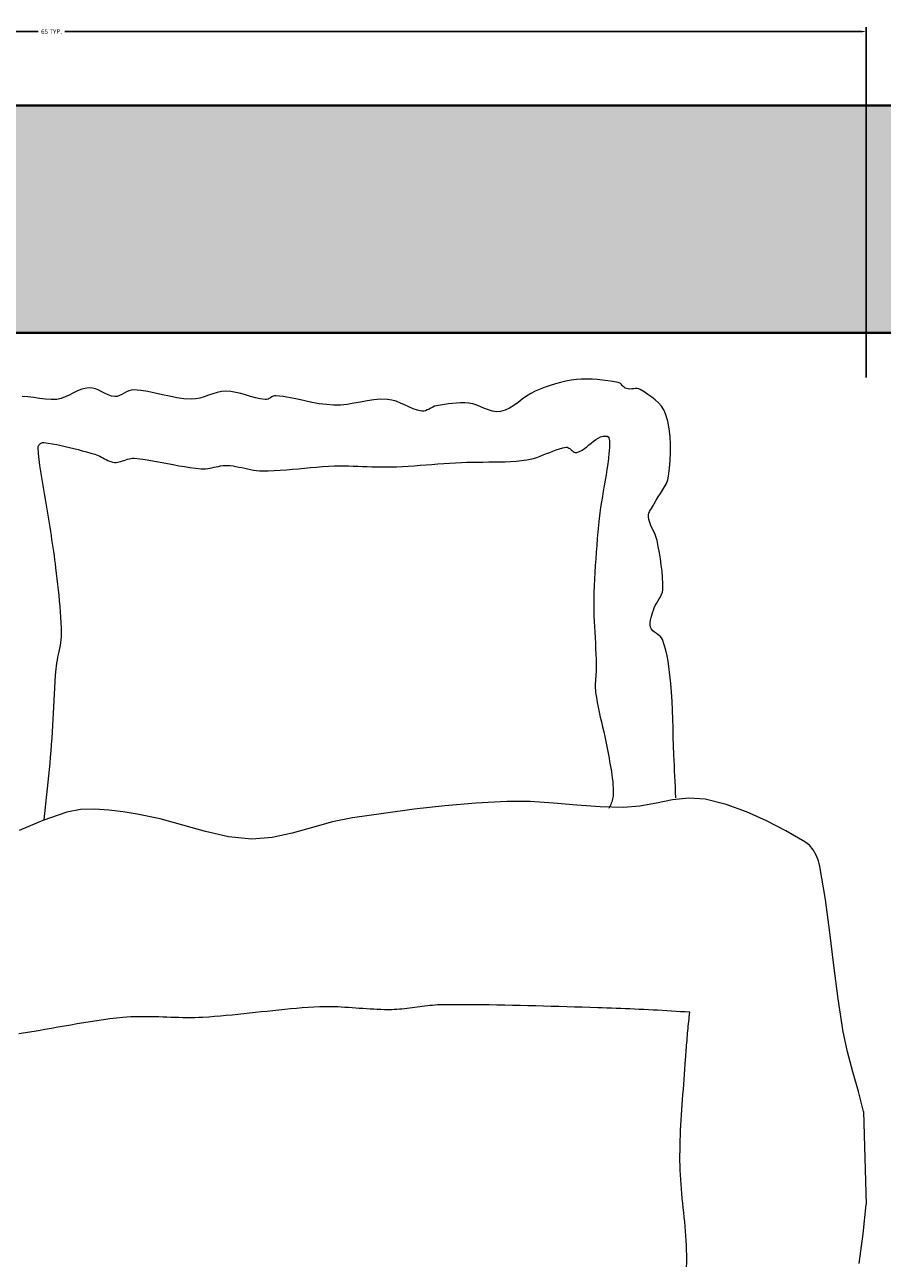
# Model space of a CAD drawing. Units: inches. Extents: x 1441 to 2460, y 1648 to 2683.
# Tile 28 of 35: x 1840 to 1874, y 2253 to 2302. Entities that reach past the tile are written whole.
import ezdxf

# ---------------------------------------------------------------- set-up
doc = ezdxf.new("R2010")
doc.units = ezdxf.units.IN
for name, color, linetype, lineweight in [('A-ANNO-DIMS', 2, 'Continuous', 18), ('A-FURN', 8, 'Continuous', 15), ('A-WALL', 7, 'Continuous', 40)]:
    doc.layers.add(name, color=color, linetype=linetype, lineweight=lineweight)
doc.layers.add('A-WALL-PATT', color=251, linetype='Continuous', lineweight=13, true_color=0x636466)
doc.styles.get("Standard").update_dxf_attribs({"font": 'arial.ttf'})
doc.dimstyles.get("Standard").update_dxf_attribs({"dimtxt": 0.18, "dimasz": 0.18, "dimexe": 0.18, "dimexo": 0.0625, "dimgap": 0.09, "dimtad": 0, "dimtih": 1, "dimtoh": 1, "dimdec": 4, "dimzin": 0, "dimdsep": 46, "dimtxsty": 'Standard', "dimcen": 0.09, "dimadec": 0, "dimazin": 0, "dimtfac": 1, "dimtdec": 4, "dimtofl": 0, "dimtmove": 0, "dimatfit": 3, "dimfxl": 1, "dimtolj": 1, "dimtzin": 0, "dimarcsym": 0})

# ---------------------------------------------------------------- blocks, each defined once
blk = doc.blocks.new('BED-DOUBLE-PLAN')
for p, q in [((53.027, 91.67), (52.818, 91.642)), ((53.234, 91.686), (53.027, 91.67)), ((53.441, 91.69), (53.234, 91.686)), ((53.649, 91.684), (53.441, 91.69)), ((53.857, 91.67), (53.649, 91.684)), ((33.253, 91.205), (33.099, 91.129)), ((33.41, 91.271), (33.253, 91.205)), ((33.569, 91.32), (33.41, 91.271)), ((33.735, 91.343), (33.569, 91.32)), ((33.867, 91.333), (33.735, 91.343)), ((33.995, 91.298), (33.867, 91.333)), ((34.121, 91.245), (33.995, 91.298)), ((34.245, 91.181), (34.121, 91.245)), ((34.37, 91.117), (34.245, 91.181)), ((35.307, 91.222), (35.216, 91.178)), ((35.4, 91.252), (35.307, 91.222)), ((35.496, 91.261), (35.4, 91.252)), ((35.784, 91.238), (35.496, 91.261)), ((36.07, 91.194), (35.784, 91.238)), ((36.354, 91.135), (36.07, 91.194)), ((38.983, 91.195), (38.81, 91.159)), ((39.158, 91.208), (38.983, 91.195)), ((39.356, 91.195), (39.158, 91.208)), ((39.551, 91.161), (39.356, 91.195)), ((51.403, 91.204), (51.224, 91.115)), ((51.599, 91.285), (51.403, 91.204)), ((51.797, 91.361), (51.599, 91.285)), ((51.997, 91.432), (51.797, 91.361)), ((52.2, 91.497), (51.997, 91.432)), ((52.404, 91.554), (52.2, 91.497)), ((52.61, 91.603), (52.404, 91.554)), ((52.818, 91.642), (52.61, 91.603)), ((54.065, 91.648), (53.857, 91.67)), ((54.272, 91.619), (54.065, 91.648)), ((54.478, 91.587), (54.272, 91.619)), ((54.683, 91.551), (54.478, 91.587)), ((54.729, 91.535), (54.683, 91.551)), ((54.771, 91.509), (54.729, 91.535)), ((54.81, 91.475), (54.771, 91.509)), ((54.847, 91.437), (54.81, 91.475)), ((54.884, 91.398), (54.847, 91.437)), ((54.922, 91.361), (54.884, 91.398)), ((54.963, 91.331), (54.922, 91.361)), ((55.008, 91.31), (54.963, 91.331)), ((55.076, 91.296), (55.008, 91.31)), ((55.147, 91.294), (55.076, 91.296)), ((55.219, 91.299), (55.147, 91.294)), ((55.292, 91.306), (55.219, 91.299)), ((55.364, 91.311), (55.292, 91.306)), ((55.433, 91.31), (55.364, 91.311)), ((55.499, 91.298), (55.433, 91.31)), ((55.56, 91.27), (55.499, 91.298)), ((55.709, 91.176), (55.56, 91.27)), ((31.32, 90.99), (31.094, 91.001)), ((31.549, 90.959), (31.32, 90.99)), ((31.78, 90.922), (31.549, 90.959)), ((32.011, 90.889), (31.78, 90.922)), ((32.24, 90.873), (32.011, 90.889)), ((32.466, 90.885), (32.24, 90.873)), ((32.63, 90.922), (32.466, 90.885)), ((32.789, 90.98), (32.63, 90.922)), ((32.945, 91.051), (32.789, 90.98)), ((33.099, 91.129), (32.945, 91.051)), ((34.495, 91.058), (34.37, 91.117)), ((34.624, 91.015), (34.495, 91.058)), ((34.756, 90.994), (34.624, 91.015)), ((34.852, 91.003), (34.756, 90.994)), ((34.945, 91.032), (34.852, 91.003)), ((35.036, 91.076), (34.945, 91.032)), ((35.126, 91.127), (35.036, 91.076)), ((35.216, 91.178), (35.126, 91.127)), ((36.638, 91.07), (36.354, 91.135)), ((36.922, 91.006), (36.638, 91.07)), ((37.206, 90.949), (36.922, 91.006)), ((37.492, 90.908), (37.206, 90.949)), ((37.78, 90.89), (37.492, 90.908)), ((37.955, 90.902), (37.78, 90.89)), ((38.128, 90.938), (37.955, 90.902)), ((38.299, 90.989), (38.128, 90.938)), ((38.469, 91.048), (38.299, 90.989)), ((38.639, 91.107), (38.469, 91.048)), ((38.81, 91.159), (38.639, 91.107)), ((39.744, 91.114), (39.551, 91.161)), ((39.936, 91.058), (39.744, 91.114)), ((40.129, 91), (39.936, 91.058)), ((40.322, 90.946), (40.129, 91)), ((40.516, 90.901), (40.322, 90.946)), ((40.713, 90.873), (40.516, 90.901)), ((40.767, 90.876), (40.713, 90.873)), ((40.821, 90.893), (40.767, 90.876)), ((40.873, 90.918), (40.821, 90.893)), ((40.924, 90.949), (40.873, 90.918)), ((40.975, 90.979), (40.924, 90.949)), ((41.027, 91.005), (40.975, 90.979)), ((41.081, 91.022), (41.027, 91.005)), ((41.135, 91.025), (41.081, 91.022)), ((41.423, 90.993), (41.135, 91.025)), ((41.708, 90.945), (41.423, 90.993)), ((41.993, 90.887), (41.708, 90.945)), ((42.277, 90.826), (41.993, 90.887)), ((42.561, 90.766), (42.277, 90.826)), ((42.845, 90.714), (42.561, 90.766)), ((43.131, 90.675), (42.845, 90.714)), ((44.218, 90.73), (43.952, 90.687)), ((44.483, 90.779), (44.218, 90.73)), ((44.748, 90.826), (44.483, 90.779)), ((45.014, 90.865), (44.748, 90.826)), ((45.28, 90.887), (45.014, 90.865)), ((45.546, 90.884), (45.28, 90.887)), ((45.723, 90.857), (45.546, 90.884)), ((45.894, 90.807), (45.723, 90.857)), ((46.062, 90.739), (45.894, 90.807)), ((46.228, 90.663), (46.062, 90.739)), ((47.967, 90.702), (47.807, 90.68)), ((48.127, 90.721), (47.967, 90.702)), ((48.287, 90.734), (48.127, 90.721)), ((48.447, 90.741), (48.287, 90.734)), ((48.607, 90.741), (48.447, 90.741)), ((48.767, 90.731), (48.607, 90.741)), ((48.926, 90.703), (48.767, 90.731)), ((49.084, 90.654), (48.926, 90.703)), ((50.723, 90.763), (50.558, 90.646)), ((50.888, 90.886), (50.723, 90.763)), ((51.053, 91.006), (50.888, 90.886)), ((51.224, 91.115), (51.053, 91.006)), ((55.86, 91.078), (55.709, 91.176)), ((56.01, 90.975), (55.86, 91.078)), ((56.153, 90.865), (56.01, 90.975)), ((56.284, 90.746), (56.153, 90.865)), ((56.399, 90.616), (56.284, 90.746)), ((43.419, 90.654), (43.131, 90.675)), ((43.686, 90.66), (43.419, 90.654)), ((43.952, 90.687), (43.686, 90.66)), ((46.394, 90.585), (46.228, 90.663)), ((46.562, 90.514), (46.394, 90.585)), ((46.733, 90.456), (46.562, 90.514)), ((46.908, 90.42), (46.733, 90.456)), ((46.984, 90.419), (46.908, 90.42)), ((47.057, 90.436), (46.984, 90.419)), ((47.128, 90.465), (47.057, 90.436)), ((47.199, 90.502), (47.128, 90.465)), ((47.27, 90.541), (47.199, 90.502)), ((47.342, 90.578), (47.27, 90.541)), ((47.415, 90.609), (47.342, 90.578)), ((47.49, 90.629), (47.415, 90.609)), ((47.648, 90.655), (47.49, 90.629)), ((47.807, 90.68), (47.648, 90.655)), ((49.24, 90.592), (49.084, 90.654)), ((49.395, 90.526), (49.24, 90.592)), ((49.549, 90.466), (49.395, 90.526)), ((49.704, 90.42), (49.549, 90.466)), ((49.861, 90.397), (49.704, 90.42)), ((50.019, 90.406), (49.861, 90.397)), ((50.209, 90.459), (50.019, 90.406)), ((50.387, 90.542), (50.209, 90.459)), ((50.558, 90.646), (50.387, 90.542)), ((56.493, 90.473), (56.399, 90.616)), ((56.561, 90.317), (56.493, 90.473)), ((56.643, 90.02), (56.561, 90.317)), ((56.701, 89.716), (56.643, 90.02)), ((56.736, 89.408), (56.701, 89.716)), ((53.616, 89.156), (53.705, 89.228)), ((53.705, 89.228), (53.796, 89.294)), ((53.796, 89.294), (53.889, 89.351)), ((53.889, 89.351), (53.985, 89.396)), ((53.985, 89.396), (54.086, 89.424)), ((54.086, 89.424), (54.192, 89.433)), ((54.192, 89.433), (54.243, 89.423)), ((54.243, 89.423), (54.282, 89.397)), ((54.282, 89.397), (54.31, 89.358)), ((54.31, 89.358), (54.329, 89.307)), ((54.329, 89.307), (54.341, 89.247)), ((54.341, 89.247), (54.346, 89.18)), ((56.752, 89.096), (56.736, 89.408)), ((31.722, 88.975), (31.723, 89)), ((31.741, 88.737), (31.722, 88.975)), ((31.723, 89), (31.729, 89.025)), ((31.729, 89.025), (31.74, 89.05)), ((31.74, 89.05), (31.755, 89.074)), ((31.765, 88.499), (31.741, 88.737)), ((31.755, 89.074), (31.774, 89.097)), ((31.774, 89.097), (31.795, 89.117)), ((31.795, 89.117), (31.818, 89.136)), ((31.818, 89.136), (31.843, 89.151)), ((31.843, 89.151), (31.869, 89.163)), ((31.869, 89.163), (31.896, 89.172)), ((31.896, 89.172), (31.922, 89.176)), ((31.922, 89.176), (31.948, 89.176)), ((31.948, 89.176), (32.119, 89.153)), ((32.119, 89.153), (32.29, 89.126)), ((32.29, 89.126), (32.459, 89.095)), ((32.459, 89.095), (32.629, 89.06)), ((32.629, 89.06), (32.797, 89.023)), ((32.797, 89.023), (32.966, 88.982)), ((32.966, 88.982), (33.133, 88.94)), ((33.133, 88.94), (33.301, 88.895)), ((33.301, 88.895), (33.468, 88.85)), ((33.468, 88.85), (33.635, 88.803)), ((33.635, 88.803), (33.801, 88.756)), ((33.801, 88.756), (33.968, 88.709)), ((51.719, 88.683), (51.846, 88.735)), ((51.846, 88.735), (51.972, 88.787)), ((51.972, 88.787), (52.1, 88.838)), ((52.1, 88.838), (52.228, 88.885)), ((52.228, 88.885), (52.357, 88.926)), ((52.357, 88.926), (52.488, 88.961)), ((52.488, 88.961), (52.621, 88.986)), ((52.621, 88.986), (52.66, 88.986)), ((52.66, 88.986), (52.697, 88.976)), ((52.697, 88.976), (52.734, 88.958)), ((52.734, 88.958), (52.769, 88.934)), ((52.769, 88.934), (52.804, 88.906)), ((52.804, 88.906), (52.839, 88.877)), ((52.839, 88.877), (52.873, 88.848)), ((52.873, 88.848), (52.908, 88.822)), ((52.908, 88.822), (52.943, 88.8)), ((52.943, 88.8), (52.979, 88.785)), ((52.979, 88.785), (53.015, 88.778)), ((53.015, 88.778), (53.053, 88.783)), ((53.053, 88.783), (53.155, 88.821)), ((53.155, 88.821), (53.253, 88.873)), ((53.253, 88.873), (53.347, 88.936)), ((53.347, 88.936), (53.438, 89.006)), ((53.438, 89.006), (53.527, 89.081)), ((53.527, 89.081), (53.616, 89.156)), ((54.315, 88.761), (54.295, 88.544)), ((54.321, 88.821), (54.315, 88.761)), ((54.328, 88.889), (54.321, 88.821)), ((54.335, 88.961), (54.328, 88.889)), ((54.342, 89.035), (54.335, 88.961)), ((54.346, 89.109), (54.342, 89.035)), ((54.346, 89.18), (54.346, 89.109)), ((56.736, 88.47), (56.751, 88.783)), ((56.751, 88.783), (56.752, 89.096)), ((31.795, 88.263), (31.765, 88.499)), ((31.829, 88.027), (31.795, 88.263)), ((33.968, 88.709), (34.034, 88.688)), ((34.034, 88.688), (34.099, 88.662)), ((34.099, 88.662), (34.162, 88.632)), ((34.162, 88.632), (34.225, 88.599)), ((34.225, 88.599), (34.288, 88.566)), ((34.288, 88.566), (34.35, 88.532)), ((34.35, 88.532), (34.413, 88.5)), ((34.413, 88.5), (34.476, 88.469)), ((34.476, 88.469), (34.54, 88.442)), ((34.54, 88.442), (34.605, 88.419)), ((34.605, 88.419), (34.671, 88.401)), ((34.671, 88.401), (34.739, 88.39)), ((34.739, 88.39), (34.805, 88.388)), ((34.805, 88.388), (34.87, 88.394)), ((34.87, 88.394), (34.935, 88.407)), ((34.935, 88.407), (35, 88.425)), ((35, 88.425), (35.064, 88.446)), ((35.064, 88.446), (35.128, 88.468)), ((35.128, 88.468), (35.193, 88.491)), ((35.193, 88.491), (35.257, 88.513)), ((35.257, 88.513), (35.322, 88.531)), ((35.322, 88.531), (35.387, 88.545)), ((35.387, 88.545), (35.452, 88.552)), ((35.452, 88.552), (35.518, 88.552)), ((35.518, 88.552), (35.741, 88.531)), ((35.741, 88.531), (35.963, 88.503)), ((35.963, 88.503), (36.184, 88.469)), ((36.184, 88.469), (36.405, 88.43)), ((36.405, 88.43), (36.626, 88.388)), ((36.626, 88.388), (36.847, 88.345)), ((36.847, 88.345), (37.067, 88.302)), ((37.067, 88.302), (37.288, 88.26)), ((37.288, 88.26), (37.509, 88.221)), ((38.86, 88.233), (38.945, 88.249)), ((38.945, 88.249), (39.031, 88.261)), ((39.031, 88.261), (39.117, 88.268)), ((39.117, 88.268), (39.203, 88.268)), ((39.203, 88.268), (39.32, 88.261)), ((39.32, 88.261), (39.437, 88.247)), ((39.437, 88.247), (39.553, 88.228)), ((43.213, 88.237), (43.451, 88.247)), ((43.451, 88.247), (43.636, 88.251)), ((43.636, 88.251), (43.822, 88.251)), ((43.822, 88.251), (44.007, 88.249)), ((44.007, 88.249), (44.192, 88.244)), ((44.192, 88.244), (44.377, 88.238)), ((46.141, 88.231), (46.375, 88.244)), ((46.375, 88.244), (46.609, 88.259)), ((46.609, 88.259), (46.842, 88.275)), ((46.842, 88.275), (47.076, 88.292)), ((47.076, 88.292), (47.309, 88.309)), ((47.309, 88.309), (47.543, 88.327)), ((47.543, 88.327), (47.776, 88.344)), ((47.776, 88.344), (48.01, 88.36)), ((48.01, 88.36), (48.243, 88.374)), ((48.243, 88.374), (48.477, 88.387)), ((48.477, 88.387), (48.693, 88.396)), ((48.693, 88.396), (48.91, 88.401)), ((48.91, 88.401), (49.126, 88.404)), ((49.126, 88.404), (49.343, 88.405)), ((49.343, 88.405), (49.56, 88.406)), ((49.56, 88.406), (49.776, 88.407)), ((49.776, 88.407), (49.993, 88.41)), ((49.993, 88.41), (50.209, 88.415)), ((50.209, 88.415), (50.425, 88.425)), ((50.425, 88.425), (50.64, 88.439)), ((50.64, 88.439), (50.855, 88.459)), ((50.855, 88.459), (51.07, 88.486)), ((51.07, 88.486), (51.203, 88.511)), ((51.203, 88.511), (51.334, 88.544)), ((51.334, 88.544), (51.463, 88.586)), ((51.463, 88.586), (51.591, 88.632)), ((51.591, 88.632), (51.719, 88.683)), ((54.269, 88.328), (54.239, 88.112)), ((54.295, 88.544), (54.269, 88.328)), ((56.709, 88.158), (56.736, 88.47)), ((31.866, 87.791), (31.829, 88.027)), ((31.905, 87.555), (31.866, 87.791)), ((37.509, 88.221), (37.73, 88.187)), ((37.73, 88.187), (37.953, 88.158)), ((37.953, 88.158), (38.176, 88.137)), ((38.176, 88.137), (38.262, 88.134)), ((38.262, 88.134), (38.347, 88.138)), ((38.347, 88.138), (38.433, 88.148)), ((38.433, 88.148), (38.518, 88.162)), ((38.518, 88.162), (38.604, 88.178)), ((38.604, 88.178), (38.689, 88.197)), ((38.689, 88.197), (38.774, 88.216)), ((38.774, 88.216), (38.86, 88.233)), ((39.553, 88.228), (39.668, 88.206)), ((39.668, 88.206), (39.783, 88.181)), ((39.783, 88.181), (39.899, 88.155)), ((39.899, 88.155), (40.014, 88.13)), ((40.014, 88.13), (40.13, 88.106)), ((40.13, 88.106), (40.245, 88.085)), ((40.245, 88.085), (40.361, 88.069)), ((40.361, 88.069), (40.478, 88.058)), ((40.478, 88.058), (40.595, 88.053)), ((40.595, 88.053), (40.833, 88.055)), ((40.833, 88.055), (41.071, 88.064)), ((41.071, 88.064), (41.309, 88.077)), ((41.309, 88.077), (41.547, 88.095)), ((41.547, 88.095), (41.785, 88.115)), ((41.785, 88.115), (42.023, 88.137)), ((42.023, 88.137), (42.261, 88.16)), ((42.261, 88.16), (42.499, 88.183)), ((42.499, 88.183), (42.737, 88.204)), ((42.737, 88.204), (42.975, 88.222)), ((42.975, 88.222), (43.213, 88.237)), ((44.377, 88.238), (44.562, 88.231)), ((44.562, 88.231), (44.748, 88.224)), ((44.748, 88.224), (44.933, 88.217)), ((44.933, 88.217), (45.118, 88.212)), ((45.118, 88.212), (45.303, 88.209)), ((45.303, 88.209), (45.488, 88.209)), ((45.488, 88.209), (45.674, 88.212)), ((45.674, 88.212), (45.907, 88.22)), ((45.907, 88.22), (46.141, 88.231)), ((54.205, 87.897), (54.169, 87.682)), ((54.239, 88.112), (54.205, 87.897)), ((56.643, 87.7), (56.674, 87.849)), ((56.674, 87.849), (56.709, 88.158)), ((31.946, 87.319), (31.905, 87.555)), ((31.988, 87.084), (31.946, 87.319)), ((54.132, 87.467), (54.094, 87.252)), ((54.169, 87.682), (54.132, 87.467)), ((56.359, 87.153), (56.444, 87.286)), ((56.444, 87.286), (56.523, 87.42)), ((56.523, 87.42), (56.591, 87.558)), ((56.591, 87.558), (56.643, 87.7)), ((32.03, 86.849), (31.988, 87.084)), ((32.071, 86.613), (32.03, 86.849)), ((54.021, 86.822), (53.988, 86.607)), ((54.057, 87.037), (54.021, 86.822)), ((54.094, 87.252), (54.057, 87.037)), ((56.114, 86.752), (56.189, 86.888)), ((56.189, 86.888), (56.272, 87.021)), ((56.272, 87.021), (56.359, 87.153)), ((32.11, 86.377), (32.071, 86.613)), ((32.146, 86.141), (32.11, 86.377)), ((53.959, 86.391), (53.934, 86.174)), ((53.988, 86.607), (53.959, 86.391)), ((55.878, 86.248), (55.881, 86.316)), ((55.881, 86.316), (55.898, 86.382)), ((55.898, 86.382), (55.925, 86.445)), ((55.925, 86.445), (55.96, 86.507)), ((55.96, 86.507), (56, 86.568)), ((56, 86.568), (56.041, 86.629)), ((56.041, 86.629), (56.08, 86.69)), ((56.08, 86.69), (56.114, 86.752)), ((32.17, 85.981), (32.146, 86.141)), ((32.195, 85.82), (32.17, 85.981)), ((32.22, 85.659), (32.195, 85.82)), ((53.907, 85.907), (53.881, 85.64)), ((53.934, 86.174), (53.907, 85.907)), ((55.897, 86.124), (55.878, 86.248)), ((55.933, 86.004), (55.897, 86.124)), ((55.98, 85.887), (55.933, 86.004)), ((56.034, 85.771), (55.98, 85.887)), ((32.245, 85.499), (32.22, 85.659)), ((32.269, 85.338), (32.245, 85.499)), ((32.294, 85.177), (32.269, 85.338)), ((53.857, 85.373), (53.834, 85.105)), ((53.881, 85.64), (53.857, 85.373)), ((56.09, 85.655), (56.034, 85.771)), ((56.144, 85.538), (56.09, 85.655)), ((56.189, 85.419), (56.144, 85.538)), ((56.221, 85.297), (56.189, 85.419)), ((56.268, 85.056), (56.221, 85.297)), ((32.318, 85.017), (32.294, 85.177)), ((32.342, 84.856), (32.318, 85.017)), ((32.364, 84.695), (32.342, 84.856)), ((53.813, 84.838), (53.793, 84.57)), ((53.834, 85.105), (53.813, 84.838)), ((56.313, 84.813), (56.268, 85.056)), ((56.355, 84.57), (56.313, 84.813)), ((32.385, 84.534), (32.364, 84.695)), ((32.406, 84.372), (32.385, 84.534)), ((32.424, 84.211), (32.406, 84.372)), ((53.793, 84.57), (53.775, 84.302)), ((56.391, 84.327), (56.355, 84.57)), ((56.42, 84.082), (56.391, 84.327)), ((32.449, 83.994), (32.424, 84.211)), ((32.474, 83.778), (32.449, 83.994)), ((53.76, 84.034), (53.746, 83.766)), ((53.775, 84.302), (53.76, 84.034)), ((56.44, 83.838), (56.42, 84.082)), ((56.45, 83.593), (56.44, 83.838)), ((32.499, 83.561), (32.474, 83.778)), ((32.524, 83.344), (32.499, 83.561)), ((32.549, 83.127), (32.524, 83.344)), ((53.735, 83.498), (53.725, 83.23)), ((53.746, 83.766), (53.735, 83.498)), ((56.432, 83.251), (56.446, 83.348)), ((56.446, 83.348), (56.45, 83.593)), ((32.571, 82.909), (32.549, 83.127)), ((32.592, 82.692), (32.571, 82.909)), ((53.719, 82.961), (53.717, 82.745)), ((53.725, 83.23), (53.719, 82.961)), ((56.194, 82.81), (56.248, 82.897)), ((56.248, 82.897), (56.304, 82.983)), ((56.304, 82.983), (56.356, 83.07)), ((56.356, 83.07), (56.4, 83.159)), ((56.4, 83.159), (56.432, 83.251)), ((32.61, 82.475), (32.592, 82.692)), ((32.625, 82.257), (32.61, 82.475)), ((53.717, 82.745), (53.719, 82.529)), ((53.719, 82.529), (53.725, 82.313)), ((56.011, 82.343), (56.043, 82.439)), ((56.043, 82.439), (56.077, 82.535)), ((56.077, 82.535), (56.108, 82.628)), ((56.108, 82.628), (56.146, 82.721)), ((56.146, 82.721), (56.194, 82.81)), ((32.637, 82.04), (32.625, 82.257)), ((32.645, 81.822), (32.637, 82.04)), ((53.725, 82.313), (53.733, 82.097)), ((53.733, 82.097), (53.743, 81.881)), ((53.743, 81.881), (53.755, 81.665)), ((55.95, 82.052), (55.961, 82.149)), ((55.951, 81.956), (55.95, 82.052)), ((55.967, 81.861), (55.951, 81.956)), ((55.961, 82.149), (55.983, 82.246)), ((55.983, 82.246), (56.011, 82.343)), ((32.635, 81.37), (32.644, 81.487)), ((32.644, 81.487), (32.648, 81.604)), ((32.648, 81.604), (32.645, 81.822)), ((53.755, 81.665), (53.768, 81.449)), ((53.768, 81.449), (53.78, 81.233)), ((56.001, 81.786), (55.967, 81.861)), ((56.055, 81.723), (56.001, 81.786)), ((56.122, 81.667), (56.055, 81.723)), ((56.197, 81.616), (56.122, 81.667)), ((56.273, 81.564), (56.197, 81.616)), ((56.343, 81.51), (56.273, 81.564)), ((56.401, 81.448), (56.343, 81.51)), ((56.441, 81.375), (56.401, 81.448)), ((32.532, 80.792), (32.556, 80.908)), ((32.556, 80.908), (32.58, 81.023)), ((32.58, 81.023), (32.602, 81.139)), ((32.602, 81.139), (32.62, 81.254)), ((32.62, 81.254), (32.635, 81.37)), ((53.78, 81.233), (53.792, 81.017)), ((53.792, 81.017), (53.803, 80.801)), ((56.51, 81.165), (56.441, 81.375)), ((56.568, 80.953), (56.51, 81.165)), ((56.617, 80.737), (56.568, 80.953)), ((32.446, 80.329), (32.463, 80.445)), ((32.463, 80.445), (32.484, 80.561)), ((32.484, 80.561), (32.507, 80.677)), ((32.507, 80.677), (32.532, 80.792)), ((53.803, 80.801), (53.812, 80.585)), ((53.812, 80.585), (53.817, 80.369)), ((56.657, 80.52), (56.617, 80.737)), ((56.691, 80.301), (56.657, 80.52)), ((32.394, 79.715), (32.412, 79.964)), ((32.412, 79.964), (32.433, 80.213)), ((32.433, 80.213), (32.446, 80.329)), ((53.796, 79.916), (53.789, 79.825)), ((53.803, 80.007), (53.796, 79.916)), ((53.81, 80.097), (53.803, 80.007)), ((53.815, 80.188), (53.81, 80.097)), ((53.817, 80.278), (53.815, 80.188)), ((53.817, 80.369), (53.817, 80.278)), ((56.72, 80.081), (56.691, 80.301)), ((56.745, 79.861), (56.72, 80.081)), ((32.365, 79.217), (32.379, 79.466)), ((32.379, 79.466), (32.394, 79.715)), ((53.778, 79.644), (53.776, 79.554)), ((53.776, 79.554), (53.776, 79.464)), ((53.776, 79.464), (53.781, 79.374)), ((53.782, 79.735), (53.778, 79.644)), ((53.789, 79.825), (53.782, 79.735)), ((56.767, 79.641), (56.745, 79.861)), ((56.798, 79.289), (56.767, 79.641)), ((32.341, 78.718), (32.353, 78.967)), ((32.353, 78.967), (32.365, 79.217)), ((53.781, 79.374), (53.791, 79.284)), ((53.791, 79.284), (53.819, 79.088)), ((53.819, 79.088), (53.853, 78.892)), ((56.82, 78.937), (56.798, 79.289)), ((56.836, 78.584), (56.82, 78.937)), ((32.318, 78.219), (32.33, 78.469)), ((32.33, 78.469), (32.341, 78.718)), ((53.853, 78.892), (53.891, 78.697)), ((53.891, 78.697), (53.932, 78.503)), ((53.932, 78.503), (53.975, 78.309)), ((56.848, 78.231), (56.836, 78.584)), ((32.291, 77.721), (32.305, 77.97)), ((32.305, 77.97), (32.318, 78.219)), ((53.975, 78.309), (54.019, 78.115)), ((54.019, 78.115), (54.065, 77.922)), ((56.857, 77.878), (56.848, 78.231)), ((32.257, 77.223), (32.275, 77.472)), ((32.275, 77.472), (32.291, 77.721)), ((54.065, 77.922), (54.11, 77.728)), ((54.11, 77.728), (54.154, 77.534)), ((54.154, 77.534), (54.197, 77.34)), ((56.866, 77.524), (56.857, 77.878)), ((56.876, 77.171), (56.866, 77.524)), ((32.215, 76.726), (32.237, 76.974)), ((32.237, 76.974), (32.257, 77.223)), ((54.197, 77.34), (54.237, 77.145)), ((54.237, 77.145), (54.274, 76.95)), ((56.89, 76.818), (56.876, 77.171)), ((32.17, 76.23), (32.193, 76.478)), ((32.193, 76.478), (32.215, 76.726)), ((54.274, 76.95), (54.298, 76.818)), ((54.298, 76.818), (54.322, 76.686)), ((54.322, 76.686), (54.346, 76.554)), ((54.346, 76.554), (54.37, 76.421)), ((56.899, 76.605), (56.89, 76.818)), ((56.908, 76.392), (56.899, 76.605)), ((32.147, 75.981), (32.17, 76.23)), ((54.37, 76.421), (54.393, 76.289)), ((54.393, 76.289), (54.414, 76.156)), ((54.414, 76.156), (54.434, 76.023)), ((54.434, 76.023), (54.451, 75.89)), ((56.918, 76.179), (56.908, 76.392)), ((56.928, 75.966), (56.918, 76.179)), ((32.097, 75.486), (32.122, 75.733)), ((32.122, 75.733), (32.147, 75.981)), ((54.451, 75.89), (54.466, 75.757)), ((54.466, 75.757), (54.478, 75.624)), ((54.478, 75.624), (54.486, 75.49)), ((56.937, 75.753), (56.928, 75.966)), ((56.947, 75.54), (56.937, 75.753)), ((56.957, 75.327), (56.947, 75.54)), ((32.043, 74.99), (32.07, 75.238)), ((32.07, 75.238), (32.097, 75.486)), ((54.447, 75.012), (54.43, 74.957)), ((54.461, 75.069), (54.447, 75.012)), ((54.472, 75.126), (54.461, 75.069)), ((54.481, 75.184), (54.472, 75.126)), ((54.487, 75.241), (54.481, 75.184)), ((54.486, 75.49), (54.49, 75.356)), ((54.49, 75.299), (54.487, 75.241)), ((54.49, 75.356), (54.49, 75.299)), ((56.84, 75.028), (56.194, 74.904)), ((57.484, 75.097), (56.84, 75.028)), ((56.967, 75.114), (56.957, 75.327)), ((58.123, 75.053), (57.484, 75.097)), ((58.956, 74.846), (58.123, 75.053)), ((32.864, 74.545), (31.901, 74.215)), ((31.986, 74.495), (32.015, 74.742)), ((32.015, 74.742), (32.043, 74.99)), ((33.405, 74.651), (32.864, 74.545)), ((33.96, 74.67), (33.405, 74.651)), ((34.522, 74.63), (33.96, 74.67)), ((35.083, 74.555), (34.522, 74.63)), ((35.638, 74.47), (35.083, 74.555)), ((46.604, 74.657), (45.387, 74.497)), ((47.824, 74.794), (46.604, 74.657)), ((49.046, 74.901), (47.824, 74.794)), ((50.27, 74.969), (49.046, 74.901)), ((51.196, 74.964), (50.27, 74.969)), ((52.121, 74.904), (51.196, 74.964)), ((53.045, 74.821), (52.121, 74.904)), ((53.971, 74.75), (53.045, 74.821)), ((54.897, 74.726), (53.971, 74.75)), ((54.34, 74.744), (54.311, 74.694)), ((54.366, 74.795), (54.34, 74.744)), ((54.39, 74.848), (54.366, 74.795)), ((54.411, 74.902), (54.39, 74.848)), ((54.43, 74.957), (54.411, 74.902)), ((55.545, 74.784), (54.897, 74.726)), ((56.194, 74.904), (55.545, 74.784)), ((59.766, 74.555), (58.956, 74.846)), ((60.555, 74.2), (59.766, 74.555)), ((31.901, 74.215), (30.964, 73.813)), ((31.956, 74.247), (31.986, 74.495)), ((36.55, 74.284), (35.638, 74.47)), ((37.452, 74.033), (36.55, 74.284)), ((38.351, 73.775), (37.452, 74.033)), ((43.37, 74.156), (42.576, 73.933)), ((44.172, 74.323), (43.37, 74.156)), ((45.387, 74.497), (44.172, 74.323)), ((61.324, 73.8), (60.555, 74.2)), ((39.257, 73.571), (38.351, 73.775)), ((40.176, 73.479), (39.257, 73.571)), ((40.985, 73.539), (40.176, 73.479)), ((41.783, 73.709), (40.985, 73.539)), ((42.576, 73.933), (41.783, 73.709)), ((62.074, 73.372), (61.324, 73.8)), ((62.255, 73.232), (62.074, 73.372)), ((62.403, 73.052), (62.255, 73.232)), ((62.52, 72.843), (62.403, 73.052)), ((62.608, 72.619), (62.52, 72.843)), ((62.667, 72.392), (62.608, 72.619)), ((62.893, 71.092), (62.667, 72.392)), ((63.068, 69.783), (62.893, 71.092)), ((63.223, 68.471), (63.068, 69.783)), ((63.387, 67.161), (63.223, 68.471)), ((63.59, 65.856), (63.387, 67.161)), ((41.018, 66.686), (40.787, 66.661)), ((41.25, 66.711), (41.018, 66.686)), ((41.481, 66.734), (41.25, 66.711)), ((41.712, 66.756), (41.481, 66.734)), ((41.944, 66.776), (41.712, 66.756)), ((42.175, 66.795), (41.944, 66.776)), ((42.407, 66.811), (42.175, 66.795)), ((42.639, 66.825), (42.407, 66.811)), ((42.871, 66.836), (42.639, 66.825)), ((43.013, 66.84), (42.871, 66.836)), ((43.155, 66.842), (43.013, 66.84)), ((43.298, 66.841), (43.155, 66.842)), ((43.44, 66.838), (43.298, 66.841)), ((43.582, 66.833), (43.44, 66.838)), ((43.724, 66.826), (43.582, 66.833)), ((43.867, 66.819), (43.724, 66.826)), ((44.009, 66.81), (43.867, 66.819)), ((44.151, 66.8), (44.009, 66.81)), ((44.294, 66.79), (44.151, 66.8)), ((44.436, 66.78), (44.294, 66.79)), ((44.578, 66.77), (44.436, 66.78)), ((44.72, 66.76), (44.578, 66.77)), ((44.863, 66.751), (44.72, 66.76)), ((45.005, 66.743), (44.863, 66.751)), ((45.147, 66.736), (45.005, 66.743)), ((45.29, 66.731), (45.147, 66.736)), ((45.432, 66.727), (45.29, 66.731)), ((45.574, 66.726), (45.432, 66.727)), ((45.717, 66.727), (45.574, 66.726)), ((45.818, 66.73), (45.717, 66.727)), ((45.92, 66.735), (45.818, 66.73)), ((46.021, 66.742), (45.92, 66.735)), ((46.122, 66.751), (46.021, 66.742)), ((46.223, 66.761), (46.122, 66.751)), ((46.324, 66.773), (46.223, 66.761)), ((46.425, 66.785), (46.324, 66.773)), ((46.526, 66.798), (46.425, 66.785)), ((46.627, 66.811), (46.526, 66.798)), ((46.727, 66.825), (46.627, 66.811)), ((46.828, 66.839), (46.727, 66.825)), ((46.929, 66.852), (46.828, 66.839)), ((47.03, 66.865), (46.929, 66.852)), ((47.131, 66.877), (47.03, 66.865)), ((47.232, 66.888), (47.131, 66.877)), ((47.333, 66.898), (47.232, 66.888)), ((47.434, 66.906), (47.333, 66.898)), ((47.535, 66.912), (47.434, 66.906)), ((47.637, 66.917), (47.535, 66.912)), ((47.738, 66.919), (47.637, 66.917)), ((48.045, 66.921), (47.738, 66.919)), ((48.352, 66.922), (48.045, 66.921)), ((48.658, 66.921), (48.352, 66.922)), ((48.965, 66.92), (48.658, 66.921)), ((49.272, 66.917), (48.965, 66.92)), ((49.579, 66.913), (49.272, 66.917)), ((49.885, 66.909), (49.579, 66.913)), ((50.192, 66.903), (49.885, 66.909)), ((50.499, 66.897), (50.192, 66.903)), ((50.806, 66.89), (50.499, 66.897)), ((51.112, 66.883), (50.806, 66.89)), ((51.419, 66.875), (51.112, 66.883)), ((51.726, 66.866), (51.419, 66.875)), ((52.032, 66.857), (51.726, 66.866)), ((52.339, 66.848), (52.032, 66.857)), ((52.646, 66.839), (52.339, 66.848)), ((52.952, 66.83), (52.646, 66.839)), ((53.259, 66.82), (52.952, 66.83)), ((53.566, 66.811), (53.259, 66.82)), ((53.872, 66.801), (53.566, 66.811)), ((54.055, 66.796), (53.872, 66.801)), ((54.237, 66.79), (54.055, 66.796)), ((54.42, 66.783), (54.237, 66.79)), ((54.602, 66.777), (54.42, 66.783)), ((54.785, 66.77), (54.602, 66.777)), ((54.967, 66.762), (54.785, 66.77)), ((55.15, 66.755), (54.967, 66.762)), ((55.332, 66.747), (55.15, 66.755)), ((55.515, 66.738), (55.332, 66.747)), ((55.697, 66.729), (55.515, 66.738)), ((55.879, 66.72), (55.697, 66.729)), ((56.062, 66.711), (55.879, 66.72)), ((56.244, 66.701), (56.062, 66.711)), ((56.426, 66.691), (56.244, 66.701)), ((56.609, 66.681), (56.426, 66.691)), ((56.791, 66.67), (56.609, 66.681)), ((56.973, 66.659), (56.791, 66.67)), ((33.53, 66.207), (33.273, 66.163)), ((33.787, 66.248), (33.53, 66.207)), ((34.045, 66.287), (33.787, 66.248)), ((34.303, 66.324), (34.045, 66.287)), ((34.561, 66.358), (34.303, 66.324)), ((34.82, 66.388), (34.561, 66.358)), ((35.079, 66.415), (34.82, 66.388)), ((35.237, 66.428), (35.079, 66.415)), ((35.394, 66.438), (35.237, 66.428)), ((35.552, 66.444), (35.394, 66.438)), ((35.71, 66.448), (35.552, 66.444)), ((35.868, 66.45), (35.71, 66.448)), ((36.026, 66.449), (35.868, 66.45)), ((36.184, 66.447), (36.026, 66.449)), ((36.343, 66.444), (36.184, 66.447)), ((36.501, 66.439), (36.343, 66.444)), ((36.66, 66.434), (36.501, 66.439)), ((36.818, 66.428), (36.66, 66.434)), ((36.976, 66.423), (36.818, 66.428)), ((37.135, 66.418), (36.976, 66.423)), ((37.293, 66.413), (37.135, 66.418)), ((37.451, 66.41), (37.293, 66.413)), ((37.61, 66.408), (37.451, 66.41)), ((37.768, 66.408), (37.61, 66.408)), ((37.926, 66.41), (37.768, 66.408)), ((38.084, 66.414), (37.926, 66.41)), ((38.242, 66.421), (38.084, 66.414)), ((38.474, 66.435), (38.242, 66.421)), ((38.706, 66.451), (38.474, 66.435)), ((38.938, 66.47), (38.706, 66.451)), ((39.169, 66.49), (38.938, 66.47)), ((39.4, 66.512), (39.169, 66.49)), ((39.632, 66.535), (39.4, 66.512)), ((39.863, 66.56), (39.632, 66.535)), ((40.094, 66.585), (39.863, 66.56)), ((40.325, 66.61), (40.094, 66.585)), ((40.556, 66.636), (40.325, 66.61)), ((40.787, 66.661), (40.556, 66.636)), ((57.155, 66.648), (56.973, 66.659)), ((57.338, 66.636), (57.155, 66.648)), ((57.52, 66.624), (57.338, 66.636)), ((57.469, 66.161), (57.479, 66.254)), ((57.479, 66.254), (57.489, 66.346)), ((57.489, 66.346), (57.499, 66.439)), ((57.499, 66.439), (57.509, 66.531)), ((57.509, 66.531), (57.52, 66.624)), ((31.218, 65.805), (30.96, 65.765)), ((31.475, 65.847), (31.218, 65.805)), ((31.732, 65.891), (31.475, 65.847)), ((31.989, 65.936), (31.732, 65.891)), ((32.246, 65.982), (31.989, 65.936)), ((32.502, 66.028), (32.246, 65.982)), ((32.759, 66.074), (32.502, 66.028)), ((33.016, 66.119), (32.759, 66.074)), ((33.273, 66.163), (33.016, 66.119)), ((57.416, 65.606), (57.425, 65.699)), ((57.425, 65.699), (57.433, 65.791)), ((57.433, 65.791), (57.442, 65.884)), ((57.442, 65.884), (57.451, 65.976)), ((57.451, 65.976), (57.46, 66.069)), ((57.46, 66.069), (57.469, 66.161)), ((63.763, 65.061), (63.59, 65.856)), ((57.378, 65.142), (57.385, 65.235)), ((57.385, 65.235), (57.393, 65.328)), ((57.393, 65.328), (57.4, 65.421)), ((57.4, 65.421), (57.408, 65.513)), ((57.408, 65.513), (57.416, 65.606)), ((57.338, 64.57), (57.352, 64.771)), ((57.352, 64.771), (57.358, 64.864)), ((57.358, 64.864), (57.364, 64.957)), ((57.364, 64.957), (57.371, 65.05)), ((57.371, 65.05), (57.378, 65.142)), ((63.975, 64.273), (63.763, 65.061)), ((57.309, 64.168), (57.324, 64.369)), ((57.324, 64.369), (57.338, 64.57)), ((64.196, 63.488), (63.975, 64.273)), ((57.263, 63.566), (57.278, 63.767)), ((57.278, 63.767), (57.294, 63.968)), ((57.294, 63.968), (57.309, 64.168)), ((57.233, 63.164), (57.248, 63.365)), ((57.248, 63.365), (57.263, 63.566)), ((64.395, 62.698), (64.196, 63.488)), ((57.191, 62.56), (57.204, 62.762)), ((57.204, 62.762), (57.218, 62.963)), ((57.218, 62.963), (57.233, 63.164)), ((57.168, 62.158), (57.179, 62.359)), ((57.179, 62.359), (57.191, 62.56)), ((64.395, 62.698), (64.503, 59.019)), ((57.149, 61.756), (57.157, 61.957)), ((57.157, 61.957), (57.168, 62.158)), ((57.132, 61.152), (57.136, 61.353)), ((57.136, 61.353), (57.141, 61.555)), ((57.141, 61.555), (57.149, 61.756)), ((57.13, 60.951), (57.132, 61.152)), ((57.13, 60.749), (57.13, 60.951)), ((57.133, 60.563), (57.13, 60.749)), ((57.139, 60.376), (57.133, 60.563)), ((57.147, 60.19), (57.139, 60.376)), ((57.159, 60.003), (57.147, 60.19)), ((57.172, 59.817), (57.159, 60.003)), ((57.188, 59.631), (57.172, 59.817)), ((57.205, 59.445), (57.188, 59.631)), ((57.222, 59.259), (57.205, 59.445)), ((57.241, 59.073), (57.222, 59.259)), ((57.26, 58.887), (57.241, 59.073)), ((57.279, 58.701), (57.26, 58.887)), ((64.382, 57.848), (64.503, 59.019)), ((57.298, 58.515), (57.279, 58.701)), ((57.317, 58.328), (57.298, 58.515)), ((57.334, 58.142), (57.317, 58.328)), ((57.35, 57.956), (57.334, 58.142)), ((57.364, 57.77), (57.35, 57.956)), ((64.222, 56.681), (64.382, 57.848)), ((57.377, 57.584), (57.364, 57.77)), ((57.387, 57.397), (57.377, 57.584)), ((57.394, 57.211), (57.387, 57.397)), ((57.398, 57.024), (57.394, 57.211)), ((57.399, 56.865), (57.398, 57.024)), ((57.398, 56.707), (57.399, 56.865)), ((57.394, 56.548), (57.398, 56.707))]:
    blk.add_line(p, q)
blk = doc.blocks.new('*D23')
at = {"layer": 'A-ANNO-DIMS', "color": 0, "lineweight": -2, "transparency": 16777216}
for p, q in [((1809.202, 2287.933), (1809.202, 2301.803)), ((1809.382, 2301.623), (1840.924, 2301.623)), ((1873.523, 2301.623), (1841.981, 2301.623)), ((1873.703, 2287.933), (1873.703, 2301.803))]:
    blk.add_line(p, q, dxfattribs=at)
at = {"layer": 'A-ANNO-DIMS', "color": 0, "transparency": 16777216}
for points in [[(1809.382, 2301.653), (1809.382, 2301.593), (1809.202, 2301.623)], [(1873.523, 2301.653), (1873.523, 2301.593), (1873.703, 2301.623)]]:
    blk.add_solid(points, dxfattribs=at)
at = {"layer": 'Defpoints', "color": 0, "transparency": 16777216}
for p in [(1873.703, 2301.623), (1809.202, 2287.87), (1873.703, 2287.87)]:
    blk.add_point(p, dxfattribs=at)
at = {"layer": 'A-ANNO-DIMS', "color": 0, "transparency": 16777216, "insert": (1841.452, 2301.623), "char_height": 0.18, "attachment_point": 5}
blk.add_mtext('\\A1;65 TYP.', dxfattribs=at)
blk = doc.blocks.new('*D67')
at = {"layer": 'A-ANNO-DIMS', "color": 0, "lineweight": -2, "transparency": 16777216}
for p, q in [((1889.448, 2298.695), (1916.216, 2298.695)), ((1916.036, 2298.515), (1916.036, 2055.938)), ((1916.036, 1812.997), (1916.036, 2055.574)), ((1758.224, 1812.817), (1916.216, 1812.817))]:
    blk.add_line(p, q, dxfattribs=at)
at = {"layer": 'A-ANNO-DIMS', "color": 0, "transparency": 16777216}
for points in [[(1916.006, 2298.515), (1916.066, 2298.515), (1916.036, 2298.695)], [(1916.006, 1812.997), (1916.066, 1812.997), (1916.036, 1812.817)]]:
    blk.add_solid(points, dxfattribs=at)
at = {"layer": 'Defpoints', "color": 0, "transparency": 16777216}
for p in [(1889.386, 2298.695), (1916.036, 2298.695), (1758.161, 1812.817)]:
    blk.add_point(p, dxfattribs=at)
at = {"layer": 'A-ANNO-DIMS', "color": 0, "transparency": 16777216, "insert": (1916.036, 2055.756), "char_height": 0.18, "attachment_point": 5}
blk.add_mtext('\\A1;485.9', dxfattribs=at)

msp = doc.modelspace()

# ---------------------------------------------------------------- hatches: boundary and pattern name
at = {"layer": 'A-WALL-PATT'}
h = msp.add_hatch(color=256, dxfattribs=at)
h.dxf.hatch_style = 1
h.paths.add_polyline_path([(1627.5085, 2298.6952), (1568.8859, 2298.6952), (1568.8859, 2246.9605), (1577.8859, 2246.9605), (1577.8859, 2289.6952), (1627.5085, 2289.6952), (1627.5085, 2294.1952)])
h.paths.add_polyline_path([(1675.5777, 2298.6952), (1651.5085, 2298.6952), (1651.5085, 2289.6952), (1675.5777, 2289.6952), (1675.5777, 2294.1952)])
h.paths.add_polyline_path([(1667.3859, 2289.6952), (1662.8859, 2289.6952), (1662.8859, 2233.0622), (1667.3859, 2233.0622)])
h.paths.add_polyline_path([(1715.8721, 2294.3362), (1715.8721, 2295.2788), (1715.8721, 2298.6952), (1699.5777, 2298.6952), (1699.5777, 2289.6952), (1715.8721, 2289.6952)])
h.paths.add_polyline_path([(1707.8859, 2289.6952), (1703.3859, 2289.6952), (1703.3859, 2199.6952), (1707.8859, 2199.6952)])
h.paths.add_polyline_path([(1760.3859, 2204.637), (1755.8859, 2204.637), (1755.8859, 2199.6952), (1667.3859, 2199.6952), (1667.3859, 2204.637), (1662.8859, 2204.637), (1662.8859, 2195.1952), (1760.3859, 2195.1952)])
h.paths.add_polyline_path([(1760.3859, 2289.6952), (1755.8859, 2289.6952), (1755.8859, 2233.0622), (1760.3859, 2233.0622)])
h.paths.add_polyline_path([(1889.3859, 2298.6952), (1739.8721, 2298.6952), (1739.8721, 2289.6952), (1880.3859, 2289.6952), (1880.3859, 2250.8051), (1889.3859, 2250.8051)])
h.paths.add_polyline_path([(1889.3859, 2202.8051), (1880.3859, 2202.8051), (1880.3859, 2157.6952), (1747.948, 2157.6952), (1747.948, 2153.1952), (1755.8859, 2153.1952), (1755.8859, 2058.005), (1760.3859, 2058.005), (1760.3859, 2153.1952), (1880.3859, 2153.1952), (1880.3859, 2124.108), (1889.3859, 2124.108)])
h.paths.add_polyline_path([(1889.3859, 1984.8305), (1880.3859, 1984.8305), (1880.3859, 1834.1952), (1889.3859, 1834.1952)])
h.paths.add_polyline_path([(1889.3859, 2076.108), (1880.3859, 2076.108), (1880.3859, 2008.8305), (1889.3859, 2008.8305)])
h.paths.add_polyline_path([(1880.3859, 2027.1952), (1800.8859, 2027.1952), (1800.8859, 2000.9452), (1805.3859, 2000.9452), (1805.3859, 2022.6952), (1880.3859, 2022.6952)])
h.paths.add_polyline_path([(1800.8859, 2027.1952), (1760.3859, 2027.1952), (1760.3859, 2030.7912), (1755.8859, 2030.7912), (1755.8859, 2022.6952), (1800.8859, 2022.6952)])
h.paths.add_polyline_path([(1880.3859, 1974.6952), (1805.3859, 1974.6952), (1805.3859, 1978.7973), (1800.8859, 1978.7973), (1800.8859, 1974.6952), (1794.8823, 1974.6952), (1794.8823, 1970.1952), (1800.8859, 1970.1952), (1805.3859, 1970.1952), (1880.3859, 1970.1952)])
h.paths.add_polyline_path([(1760.3859, 1974.6952), (1755.8859, 1974.6952), (1755.8859, 1925.6952), (1751.8616, 1925.6952), (1751.8616, 1921.1952), (1760.3859, 1921.1952)])
h.paths.add_polyline_path([(1760.3859, 1921.1952), (1755.8859, 1921.1952), (1755.8859, 1843.1952), (1760.3859, 1843.1952)])
h.paths.add_polyline_path([(1799.1136, 1838.6952), (1799.1136, 1843.1952), (1760.3859, 1843.1952), (1751.8944, 1843.1952), (1751.8944, 1834.1952), (1758.1615, 1834.1952), (1799.1136, 1834.1952)])
h.paths.add_polyline_path([(1880.3859, 1843.1952), (1859.1136, 1843.1952), (1859.1136, 1834.1952), (1880.3859, 1834.1952)])
h.paths.add_polyline_path([(1577.8859, 1857.7914), (1568.8859, 1857.7914), (1568.8859, 1834.1952), (1695.0034, 1834.1952), (1695.0034, 1838.6952), (1695.0034, 1843.1952), (1577.8859, 1843.1952)])
h.paths.add_polyline_path([(1577.8859, 1959.2399), (1573.3859, 1959.2399), (1568.8859, 1959.2399), (1568.8859, 1905.7914), (1577.8859, 1905.7914), (1577.8859, 1921.1952), (1703.3859, 1921.1952), (1707.8859, 1921.1952), (1715.1501, 1921.1952), (1715.1501, 1925.6952), (1707.8859, 1925.6952), (1703.3859, 1925.6952), (1577.8859, 1925.6952)])
h.paths.add_polyline_path([(1577.8859, 2106.6907), (1568.8859, 2106.6907), (1568.8859, 2019.2399), (1577.8859, 2019.2399)])
h.paths.add_polyline_path([(1707.8859, 2051.6952), (1703.3859, 2051.6952), (1703.3859, 2048.6952), (1703.3859, 1925.6952), (1707.8859, 1925.6952)])
h.paths.add_polyline_path([(1703.3859, 2051.6952), (1676.3859, 2051.6952), (1676.3859, 2048.6952), (1703.3859, 2048.6952)])
h.paths.add_polyline_path([(1703.3859, 2102.6952), (1676.3859, 2102.6952), (1676.3859, 2099.6952), (1685.3859, 2099.6952), (1703.3859, 2099.6952)])
h.paths.add_polyline_path([(1707.8859, 2153.1952), (1710.5611, 2153.1952), (1710.5611, 2157.6952), (1707.8859, 2157.6952), (1707.8859, 2195.1952), (1703.3859, 2195.1952), (1703.3859, 2099.6952), (1707.8859, 2099.6952)])
h.paths.add_polyline_path([(1577.8859, 2198.9605), (1568.8859, 2198.9605), (1568.8859, 2166.6907), (1577.8859, 2166.6907)])

# ---------------------------------------------------------------- linework, layer by layer
at = {"layer": 'A-WALL'}
for p, q in [((1568.8859, 2298.6952), (1889.3859, 2298.6952)), ((1577.8859, 2289.6952), (1880.3859, 2289.6952))]:
    msp.add_line(p, q, dxfattribs=at)

# ---------------------------------------------------------------- block references
at = {"layer": 'A-FURN'}
msp.add_blockref('BED-DOUBLE-PLAN', (1809.2, 2196.18), dxfattribs=at)

# ---------------------------------------------------------------- dimensions: what is measured, and where the dimension line sits
at = {"layer": 'A-ANNO-DIMS'}
dim = msp.add_linear_dim(base=(1873.7028, 2301.6233), p1=(1809.2021, 2287.8701), p2=(1873.7028, 2287.8701), text='<> TYP.', dimstyle='Standard', override={"dimdec": 0, "dimlfac": 1, "dimrnd": 0, "dimzin": 0, "dimdsep": 46, "dimlunit": 2}, dxfattribs=at)
dim.commit()
dim.dimension.update_dxf_attribs({"geometry": '*D23', "text_midpoint": (1841.4525, 2301.6233)})
dim = msp.add_linear_dim(base=(1916.0359, 2298.6952), p1=(1758.1615, 1812.8171), p2=(1889.3859, 2298.6952), angle=90, dimstyle='Standard', override={"dimdec": 1, "dimlfac": 1, "dimrnd": 0, "dimzin": 0, "dimdsep": 46, "dimlunit": 2}, dxfattribs=at)
dim.commit()
dim.dimension.update_dxf_attribs({"geometry": '*D67', "text_midpoint": (1916.0359, 2055.7561)})

doc.saveas('drawing.dxf')
